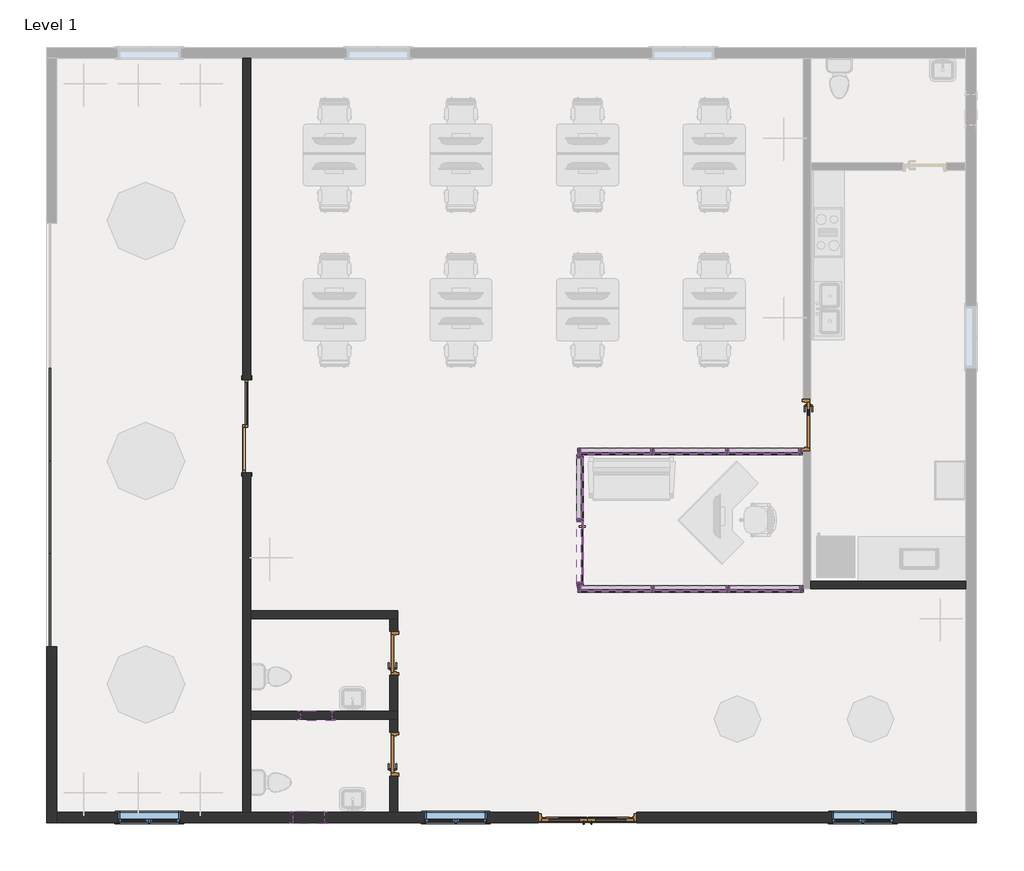
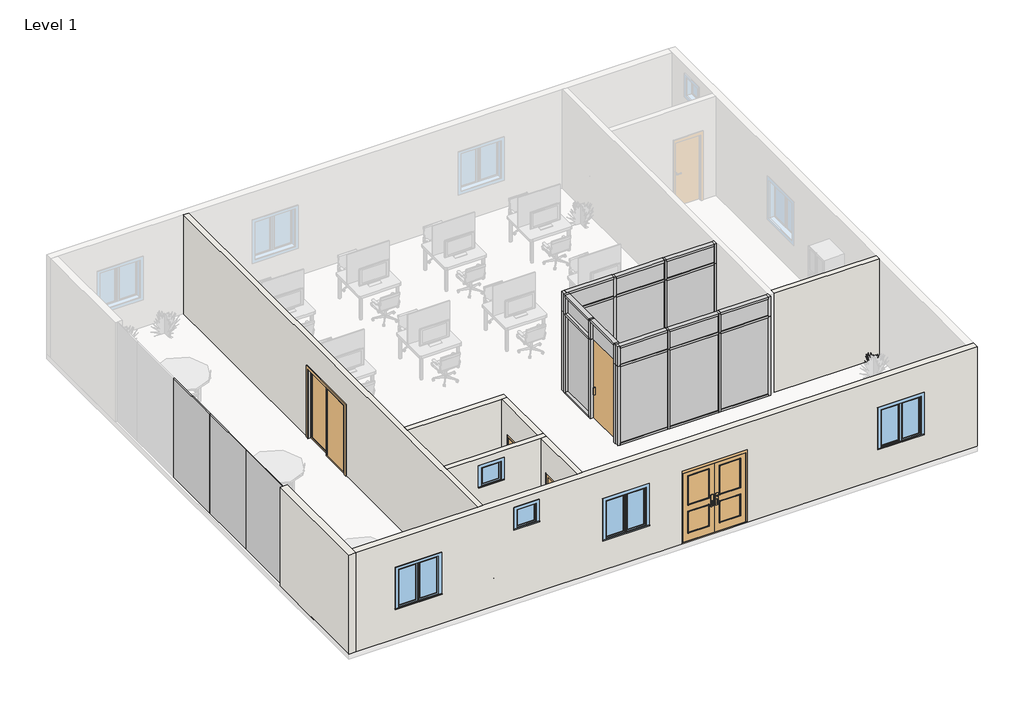
# One storey, part 1 of 2: 44 members, 18 plates, 8 walls, 6 doors, 5 windows.
"""IFC4 building model written with IfcOpenShell, lengths in millimetres."""

from ifc_helpers import new_model, si_unit, frame, origin, origin_with_axes, place, context, project, spatial, polyline, outline, extrude, faceted_brep, transform, mapped, element, save
from components import door_curtain_wall_single_glass_door_curtain_wall_single_8a977710, door_b43bda57, door_6260e01d, door_549a8064, door_95a5efb1, door_bb4af967, door_1568ef6f, member_79cc3911, member_243ec899, member_4dc7c44e, member_7022ac76, member_f0fea5a5, member_6e77e263, member_ee409385, member_47bfaf8a, member_e1cf819f, member_4b717c4e, member_f7ba7797, member_7354043d, member_7f33020a, member_c704a0f7, system_panel_glazed_acd1c6f8, system_panel_glazed_c99c457a, system_panel_glazed_58f29689, system_panel_glazed_e44632c1, system_panel_glazed_4b614736, system_panel_glazed_1dbb284f, system_panel_glazed_fd42546f, system_panel_glazed_94232cd9, system_panel_glazed_3d3fe78f, system_panel_glazed_8a2d2adf, system_panel_glazed_e91e0514, system_panel_glazed_5475d124, window_0862ab64, window_e41d21a6, window_3d781103

model = new_model("IFC4")

# Units and contexts
model_context = context("Model", 3, world=origin())
ifc_project = project(units=[si_unit("LENGTHUNIT", "METRE", prefix="MILLI")], contexts=[model_context])

# Site, building, storey
site = spatial("IfcSite", under=ifc_project)
building = spatial("IfcBuilding", under=site)
storey = spatial("IfcBuildingStorey", under=building, Name="Level 1", Elevation=0.0)

# Doors
placement = place(None, origin())
door_curtain_wall_single_glass_door_curtain_wall_single_shape = door_curtain_wall_single_glass_door_curtain_wall_single_8a977710(model_context)
element("IfcDoor", 1, ObjectType="Door-Curtain-Wall-Single-Glass : Door-Curtain-Wall-Single-Glass", at=placement, inside=storey, context=model_context, shape_type="MappedRepresentation", body=[
    mapped(door_curtain_wall_single_glass_door_curtain_wall_single_shape, transform((-9796.2738969, -3317.2711575, 0.0), x_axis=(0.0, -1.0, 0.0), y_axis=(1.0, 0.0, 0.0), z_axis=(0.0, 0.0, 1.0))),
])
door_shape = door_b43bda57(model_context)
element("IfcDoor", 2, ObjectType="Door-Double-Sliding : 72\" x 84\"", at=placement, inside=storey, context=model_context, shape_type="MappedRepresentation", body=[
    mapped(door_shape, transform((-16228.8238969, -839.1836575, 0.0), x_axis=(0.0, 1.0, 0.0), y_axis=(-1.0, 0.0, 0.0), z_axis=(0.0, 0.0, 1.0))),
])
door_2_shape = door_6260e01d(model_context)
door_3_shape = door_549a8064(model_context)
door_4_shape = door_95a5efb1(model_context)
element("IfcDoor", 3, ObjectType="Door-Exterior-Double-Two_Lite : 72\" x 84\"", at=placement, inside=storey, context=model_context, shape_type="MappedRepresentation", body=[
    mapped(door_2_shape, transform((-9650.2238969, -8529.0336575, 0.0), x_axis=(-1.0, 0.0, 0.0), y_axis=(0.0, -1.0, 0.0), z_axis=(0.0, 0.0, 1.0))),
    mapped(door_3_shape, transform((-9650.2238969, -8529.0336575, 0.0), x_axis=(-1.0, 0.0, 0.0), y_axis=(0.0, -1.0, 0.0), z_axis=(0.0, 0.0, 1.0))),
    mapped(door_4_shape, transform((-9650.2238969, -8529.0336575, 0.0), x_axis=(-1.0, 0.0, 0.0), y_axis=(0.0, -1.0, 0.0), z_axis=(0.0, 0.0, 1.0))),
])
door_5_shape = door_bb4af967(model_context)
element("IfcDoor", 4, ObjectType="Door-Passage-Single-Flush : 30\" x 80\"", at=placement, inside=storey, context=model_context, shape_type="MappedRepresentation", body=[
    mapped(door_5_shape, transform((-13453.8738969, -5309.5836575, 0.0), x_axis=(0.0, 1.0, 0.0), y_axis=(-1.0, 0.0, 0.0), z_axis=(0.0, 0.0, 1.0))),
])
element("IfcDoor", 5, ObjectType="Door-Passage-Single-Flush : 30\" x 80\"", at=placement, inside=storey, context=model_context, shape_type="MappedRepresentation", body=[
    mapped(door_5_shape, transform((-13453.8738969, -7290.7836575, 0.0), x_axis=(0.0, 1.0, 0.0), y_axis=(-1.0, 0.0, 0.0), z_axis=(0.0, 0.0, 1.0))),
])
door_6_shape = door_1568ef6f(model_context)
element("IfcDoor", 6, ObjectType="Door-Passage-Single-Two_Lite_Narrow : 36\" x 84\"", at=placement, inside=storey, context=model_context, shape_type="MappedRepresentation", body=[
    mapped(door_6_shape, transform((-5338.5738969, -813.7836575, 0.0), x_axis=(0.0, -1.0, 0.0), y_axis=(1.0, 0.0, 0.0), z_axis=(0.0, 0.0, 1.0))),
])

# Members
member_shape = member_79cc3911(model_context)
element("IfcMember", 7, ObjectType="Rectangular Mullion : 2.5\" x 5\" rectangular", at=placement, inside=storey, context=model_context, shape_type="MappedRepresentation", body=[
    mapped(member_shape, transform((-9783.5738969, -1340.8336575, 3048.0), x_axis=(0.0, 0.0, 1.0), y_axis=(0.0, 1.0, 0.0), z_axis=(-1.0, 0.0, 0.0))),
])
element("IfcMember", 8, ObjectType="Rectangular Mullion : 2.5\" x 5\" rectangular", at=placement, inside=storey, context=model_context, shape_type="MappedRepresentation", body=[
    mapped(member_shape, transform((-6868.9238969, -1340.8336575, 3048.0), x_axis=(0.0, 0.0, 1.0), y_axis=(0.0, 1.0, 0.0), z_axis=(-1.0, 0.0, 0.0))),
])
member_2_shape = member_243ec899(model_context)
element("IfcMember", 9, ObjectType="Rectangular Mullion : 2.5\" x 5\" rectangular", at=placement, inside=storey, context=model_context, shape_type="MappedRepresentation", body=[
    mapped(member_2_shape, transform((-8342.1238969, -1340.8336575, 3048.0), x_axis=(0.0, 0.0, 1.0), y_axis=(0.0, 1.0, 0.0), z_axis=(-1.0, 0.0, 0.0))),
])
element("IfcMember", 10, ObjectType="Rectangular Mullion : 2.5\" x 5\" rectangular", at=placement, inside=storey, context=model_context, shape_type="MappedRepresentation", body=[
    mapped(member_shape, transform((-5490.9738969, -1340.8336575, 0.0), x_axis=(0.0, 0.0, -1.0), y_axis=(0.0, 1.0, 0.0), z_axis=(1.0, 0.0, 0.0))),
])
element("IfcMember", 11, ObjectType="Rectangular Mullion : 2.5\" x 5\" rectangular", at=placement, inside=storey, context=model_context, shape_type="MappedRepresentation", body=[
    mapped(member_shape, transform((-8405.6238969, -1340.8336575, 0.0), x_axis=(0.0, 0.0, -1.0), y_axis=(0.0, 1.0, 0.0), z_axis=(1.0, 0.0, 0.0))),
])
element("IfcMember", 12, ObjectType="Rectangular Mullion : 2.5\" x 5\" rectangular", at=placement, inside=storey, context=model_context, shape_type="MappedRepresentation", body=[
    mapped(member_2_shape, transform((-6932.4238969, -1340.8336575, 0.0), x_axis=(0.0, 0.0, -1.0), y_axis=(0.0, 1.0, 0.0), z_axis=(1.0, 0.0, 0.0))),
])
member_3_shape = member_4dc7c44e(model_context)
element("IfcMember", 13, ObjectType="Rectangular Mullion : 2.5\" x 5\" rectangular", at=placement, inside=storey, context=model_context, shape_type="MappedRepresentation", body=[
    mapped(member_3_shape, transform((-6868.9238969, -1340.8336575, 2438.4), x_axis=(0.0, 0.0, 1.0), y_axis=(0.0, 1.0, 0.0), z_axis=(-1.0, 0.0, 0.0))),
])
element("IfcMember", 14, ObjectType="Rectangular Mullion : 2.5\" x 5\" rectangular", at=placement, inside=storey, context=model_context, shape_type="MappedRepresentation", body=[
    mapped(member_3_shape, transform((-9783.5738969, -1340.8336575, 2438.4), x_axis=(0.0, 0.0, 1.0), y_axis=(0.0, 1.0, 0.0), z_axis=(-1.0, 0.0, 0.0))),
])
member_4_shape = member_7022ac76(model_context)
element("IfcMember", 15, ObjectType="Rectangular Mullion : 2.5\" x 5\" rectangular", at=placement, inside=storey, context=model_context, shape_type="MappedRepresentation", body=[
    mapped(member_4_shape, transform((-8342.1238969, -1340.8336575, 2438.4), x_axis=(0.0, 0.0, 1.0), y_axis=(0.0, 1.0, 0.0), z_axis=(-1.0, 0.0, 0.0))),
])
member_5_shape = member_f0fea5a5(model_context)
element("IfcMember", 16, ObjectType="Rectangular Mullion : 2.5\" x 5\" rectangular", at=placement, inside=storey, context=model_context, shape_type="MappedRepresentation", body=[
    mapped(member_5_shape, transform((-6900.6738969, -1340.8336575, 0.0), x_axis=(-1.0, 0.0, 0.0), y_axis=(0.0, 1.0, 0.0), z_axis=(0.0, 0.0, -1.0))),
])
element("IfcMember", 17, ObjectType="Rectangular Mullion : 2.5\" x 5\" rectangular", at=placement, inside=storey, context=model_context, shape_type="MappedRepresentation", body=[
    mapped(member_5_shape, transform((-8373.8738969, -1340.8336575, 0.0), x_axis=(-1.0, 0.0, 0.0), y_axis=(0.0, 1.0, 0.0), z_axis=(0.0, 0.0, -1.0))),
])
element("IfcMember", 18, ObjectType="Rectangular Mullion : 2.5\" x 5\" rectangular", at=placement, inside=storey, context=model_context, shape_type="MappedRepresentation", body=[
    mapped(member_5_shape, transform((-6887.9738969, -4039.5836575, 0.0), x_axis=(-1.0, 0.0, 0.0), y_axis=(0.0, 1.0, 0.0), z_axis=(0.0, 0.0, -1.0))),
])
element("IfcMember", 19, ObjectType="Rectangular Mullion : 2.5\" x 5\" rectangular", at=placement, inside=storey, context=model_context, shape_type="MappedRepresentation", body=[
    mapped(member_5_shape, transform((-8367.5238969, -4039.5836575, 0.0), x_axis=(-1.0, 0.0, 0.0), y_axis=(0.0, 1.0, 0.0), z_axis=(0.0, 0.0, -1.0))),
])
element("IfcMember", 20, ObjectType="Rectangular Mullion : 2.5\" x 5\" rectangular", at=placement, inside=storey, context=model_context, shape_type="MappedRepresentation", body=[
    mapped(member_5_shape, transform((-9796.2738969, -2690.2086575, 0.0), x_axis=(0.0, -1.0, 0.0), y_axis=(-1.0, 0.0, 0.0), z_axis=(0.0, 0.0, -1.0))),
])
member_6_shape = member_6e77e263(model_context)
element("IfcMember", 21, ObjectType="Rectangular Mullion : 2.5\" x 5\" rectangular", at=placement, inside=storey, context=model_context, shape_type="MappedRepresentation", body=[
    mapped(member_6_shape, transform((-6900.6738969, -1340.8336575, 2438.4), x_axis=(-1.0, 0.0, 0.0), y_axis=(0.0, 1.0, 0.0), z_axis=(0.0, 0.0, -1.0))),
])
element("IfcMember", 22, ObjectType="Rectangular Mullion : 2.5\" x 5\" rectangular", at=placement, inside=storey, context=model_context, shape_type="MappedRepresentation", body=[
    mapped(member_6_shape, transform((-8373.8738969, -1340.8336575, 2438.4), x_axis=(-1.0, 0.0, 0.0), y_axis=(0.0, 1.0, 0.0), z_axis=(0.0, 0.0, -1.0))),
])
element("IfcMember", 23, ObjectType="Rectangular Mullion : 2.5\" x 5\" rectangular", at=placement, inside=storey, context=model_context, shape_type="MappedRepresentation", body=[
    mapped(member_6_shape, transform((-6887.9738969, -4039.5836575, 2438.4), x_axis=(-1.0, 0.0, 0.0), y_axis=(0.0, 1.0, 0.0), z_axis=(0.0, 0.0, -1.0))),
])
element("IfcMember", 24, ObjectType="Rectangular Mullion : 2.5\" x 5\" rectangular", at=placement, inside=storey, context=model_context, shape_type="MappedRepresentation", body=[
    mapped(member_6_shape, transform((-8367.5238969, -4039.5836575, 2438.4), x_axis=(-1.0, 0.0, 0.0), y_axis=(0.0, 1.0, 0.0), z_axis=(0.0, 0.0, -1.0))),
])
element("IfcMember", 25, ObjectType="Rectangular Mullion : 2.5\" x 5\" rectangular", at=placement, inside=storey, context=model_context, shape_type="MappedRepresentation", body=[
    mapped(member_6_shape, transform((-9796.2738969, -2690.2086575, 2438.4), x_axis=(0.0, -1.0, 0.0), y_axis=(-1.0, 0.0, 0.0), z_axis=(0.0, 0.0, -1.0))),
])
member_7_shape = member_ee409385(model_context)
element("IfcMember", 26, ObjectType="Rectangular Mullion : 2.5\" x 5\" rectangular", at=placement, inside=storey, context=model_context, shape_type="MappedRepresentation", body=[
    mapped(member_7_shape, transform((-9847.0738969, -1340.8336575, 0.0), x_axis=(-1.0, 0.0, 0.0), y_axis=(0.0, 1.0, 0.0), z_axis=(0.0, 0.0, -1.0))),
])
element("IfcMember", 27, ObjectType="Rectangular Mullion : 2.5\" x 5\" rectangular", at=placement, inside=storey, context=model_context, shape_type="MappedRepresentation", body=[
    mapped(member_7_shape, transform((-9847.0738969, -4039.5836575, 0.0), x_axis=(-1.0, 0.0, 0.0), y_axis=(0.0, 1.0, 0.0), z_axis=(0.0, 0.0, -1.0))),
])
member_8_shape = member_47bfaf8a(model_context)
element("IfcMember", 28, ObjectType="Rectangular Mullion : 2.5\" x 5\" rectangular", at=placement, inside=storey, context=model_context, shape_type="MappedRepresentation", body=[
    mapped(member_8_shape, transform((-9847.0738969, -1340.8336575, 2438.4), x_axis=(-1.0, 0.0, 0.0), y_axis=(0.0, 1.0, 0.0), z_axis=(0.0, 0.0, -1.0))),
])
element("IfcMember", 29, ObjectType="Rectangular Mullion : 2.5\" x 5\" rectangular", at=placement, inside=storey, context=model_context, shape_type="MappedRepresentation", body=[
    mapped(member_8_shape, transform((-9847.0738969, -4039.5836575, 2438.4), x_axis=(-1.0, 0.0, 0.0), y_axis=(0.0, 1.0, 0.0), z_axis=(0.0, 0.0, -1.0))),
])
element("IfcMember", 30, ObjectType="Rectangular Mullion : 2.5\" x 5\" rectangular", at=placement, inside=storey, context=model_context, shape_type="MappedRepresentation", body=[
    mapped(member_8_shape, transform((-5427.4738969, -1340.8336575, 3048.0), x_axis=(1.0, 0.0, 0.0), y_axis=(0.0, 1.0, 0.0), z_axis=(0.0, 0.0, 1.0))),
])
element("IfcMember", 31, ObjectType="Rectangular Mullion : 2.5\" x 5\" rectangular", at=placement, inside=storey, context=model_context, shape_type="MappedRepresentation", body=[
    mapped(member_8_shape, transform((-5408.4238969, -4039.5836575, 3048.0), x_axis=(1.0, 0.0, 0.0), y_axis=(0.0, 1.0, 0.0), z_axis=(0.0, 0.0, 1.0))),
])
element("IfcMember", 32, ObjectType="Rectangular Mullion : 2.5\" x 5\" rectangular", at=placement, inside=storey, context=model_context, shape_type="MappedRepresentation", body=[
    mapped(member_8_shape, transform((-9796.2738969, -1404.3336575, 3048.0), x_axis=(0.0, 1.0, 0.0), y_axis=(-1.0, 0.0, 0.0), z_axis=(0.0, 0.0, 1.0))),
])
element("IfcMember", 33, ObjectType="Rectangular Mullion : 2.5\" x 5\" rectangular", at=placement, inside=storey, context=model_context, shape_type="MappedRepresentation", body=[
    mapped(member_7_shape, transform((-5427.4738969, -1340.8336575, 2438.4), x_axis=(1.0, 0.0, 0.0), y_axis=(0.0, 1.0, 0.0), z_axis=(0.0, 0.0, 1.0))),
])
element("IfcMember", 34, ObjectType="Rectangular Mullion : 2.5\" x 5\" rectangular", at=placement, inside=storey, context=model_context, shape_type="MappedRepresentation", body=[
    mapped(member_7_shape, transform((-5408.4238969, -4039.5836575, 2438.4), x_axis=(1.0, 0.0, 0.0), y_axis=(0.0, 1.0, 0.0), z_axis=(0.0, 0.0, 1.0))),
])
element("IfcMember", 35, ObjectType="Rectangular Mullion : 2.5\" x 5\" rectangular", at=placement, inside=storey, context=model_context, shape_type="MappedRepresentation", body=[
    mapped(member_7_shape, transform((-9796.2738969, -1404.3336575, 2438.4), x_axis=(0.0, 1.0, 0.0), y_axis=(-1.0, 0.0, 0.0), z_axis=(0.0, 0.0, 1.0))),
])
member_9_shape = member_e1cf819f(model_context)
element("IfcMember", 36, ObjectType="Rectangular Mullion : 2.5\" x 5\" rectangular", at=placement, inside=storey, context=model_context, shape_type="MappedRepresentation", body=[
    mapped(member_9_shape, transform((-9783.5738969, -4039.5836575, 3048.0), x_axis=(0.0, 0.0, 1.0), y_axis=(0.0, 1.0, 0.0), z_axis=(-1.0, 0.0, 0.0))),
])
element("IfcMember", 37, ObjectType="Rectangular Mullion : 2.5\" x 5\" rectangular", at=placement, inside=storey, context=model_context, shape_type="MappedRepresentation", body=[
    mapped(member_9_shape, transform((-6856.2238969, -4039.5836575, 3048.0), x_axis=(0.0, 0.0, 1.0), y_axis=(0.0, 1.0, 0.0), z_axis=(-1.0, 0.0, 0.0))),
])
member_10_shape = member_4b717c4e(model_context)
element("IfcMember", 38, ObjectType="Rectangular Mullion : 2.5\" x 5\" rectangular", at=placement, inside=storey, context=model_context, shape_type="MappedRepresentation", body=[
    mapped(member_10_shape, transform((-8335.7738969, -4039.5836575, 3048.0), x_axis=(0.0, 0.0, 1.0), y_axis=(0.0, 1.0, 0.0), z_axis=(-1.0, 0.0, 0.0))),
])
element("IfcMember", 39, ObjectType="Rectangular Mullion : 2.5\" x 5\" rectangular", at=placement, inside=storey, context=model_context, shape_type="MappedRepresentation", body=[
    mapped(member_9_shape, transform((-5471.9238969, -4039.5836575, 0.0), x_axis=(0.0, 0.0, -1.0), y_axis=(0.0, 1.0, 0.0), z_axis=(1.0, 0.0, 0.0))),
])
element("IfcMember", 40, ObjectType="Rectangular Mullion : 2.5\" x 5\" rectangular", at=placement, inside=storey, context=model_context, shape_type="MappedRepresentation", body=[
    mapped(member_9_shape, transform((-8399.2738969, -4039.5836575, 0.0), x_axis=(0.0, 0.0, -1.0), y_axis=(0.0, 1.0, 0.0), z_axis=(1.0, 0.0, 0.0))),
])
element("IfcMember", 41, ObjectType="Rectangular Mullion : 2.5\" x 5\" rectangular", at=placement, inside=storey, context=model_context, shape_type="MappedRepresentation", body=[
    mapped(member_10_shape, transform((-6919.7238969, -4039.5836575, 0.0), x_axis=(0.0, 0.0, -1.0), y_axis=(0.0, 1.0, 0.0), z_axis=(1.0, 0.0, 0.0))),
])
member_11_shape = member_f7ba7797(model_context)
element("IfcMember", 42, ObjectType="Rectangular Mullion : 2.5\" x 5\" rectangular", at=placement, inside=storey, context=model_context, shape_type="MappedRepresentation", body=[
    mapped(member_11_shape, transform((-6856.2238969, -4039.5836575, 2438.4), x_axis=(0.0, 0.0, 1.0), y_axis=(0.0, 1.0, 0.0), z_axis=(-1.0, 0.0, 0.0))),
])
element("IfcMember", 43, ObjectType="Rectangular Mullion : 2.5\" x 5\" rectangular", at=placement, inside=storey, context=model_context, shape_type="MappedRepresentation", body=[
    mapped(member_11_shape, transform((-9783.5738969, -4039.5836575, 2438.4), x_axis=(0.0, 0.0, 1.0), y_axis=(0.0, 1.0, 0.0), z_axis=(-1.0, 0.0, 0.0))),
])
member_12_shape = member_7354043d(model_context)
element("IfcMember", 44, ObjectType="Rectangular Mullion : 2.5\" x 5\" rectangular", at=placement, inside=storey, context=model_context, shape_type="MappedRepresentation", body=[
    mapped(member_12_shape, transform((-8335.7738969, -4039.5836575, 2438.4), x_axis=(0.0, 0.0, 1.0), y_axis=(0.0, 1.0, 0.0), z_axis=(-1.0, 0.0, 0.0))),
])
member_13_shape = member_7f33020a(model_context)
element("IfcMember", 45, ObjectType="Rectangular Mullion : 2.5\" x 5\" rectangular", at=placement, inside=storey, context=model_context, shape_type="MappedRepresentation", body=[
    mapped(member_13_shape, transform((-9796.2738969, -3912.5836575, 3048.0), x_axis=(0.0, 0.0, 1.0), y_axis=(-1.0, 0.0, 0.0), z_axis=(0.0, -1.0, 0.0))),
])
element("IfcMember", 46, ObjectType="Rectangular Mullion : 2.5\" x 5\" rectangular", at=placement, inside=storey, context=model_context, shape_type="MappedRepresentation", body=[
    mapped(member_13_shape, transform((-9796.2738969, -2658.4586575, 3048.0), x_axis=(0.0, 0.0, 1.0), y_axis=(-1.0, 0.0, 0.0), z_axis=(0.0, -1.0, 0.0))),
])
element("IfcMember", 47, ObjectType="Rectangular Mullion : 2.5\" x 5\" rectangular", at=placement, inside=storey, context=model_context, shape_type="MappedRepresentation", body=[
    mapped(member_13_shape, transform((-9796.2738969, -1467.8336575, 0.0), x_axis=(0.0, 0.0, -1.0), y_axis=(-1.0, 0.0, 0.0), z_axis=(0.0, 1.0, 0.0))),
])
member_14_shape = member_c704a0f7(model_context)
element("IfcMember", 48, ObjectType="Rectangular Mullion : 2.5\" x 5\" rectangular", at=placement, inside=storey, context=model_context, shape_type="MappedRepresentation", body=[
    mapped(member_14_shape, transform((-9796.2738969, -2658.4586575, 2438.4), x_axis=(0.0, 0.0, 1.0), y_axis=(-1.0, 0.0, 0.0), z_axis=(0.0, -1.0, 0.0))),
])
element("IfcMember", 49, ObjectType="Rectangular Mullion : 2.5\" x 5\" rectangular", at=placement, inside=storey, context=model_context, shape_type="MappedRepresentation", body=[
    mapped(member_8_shape, transform((-9796.2738969, -3976.0836575, 2438.4), x_axis=(0.0, -1.0, 0.0), y_axis=(-1.0, 0.0, 0.0), z_axis=(0.0, 0.0, -1.0))),
])
element("IfcMember", 50, ObjectType="Rectangular Mullion : 2.5\" x 5\" rectangular", at=placement, inside=storey, context=model_context, shape_type="MappedRepresentation", body=[
    mapped(member_7_shape, transform((-9796.2738969, -3976.0836575, 0.0), x_axis=(0.0, -1.0, 0.0), y_axis=(-1.0, 0.0, 0.0), z_axis=(0.0, 0.0, -1.0))),
])

# Plates
system_panel_glazed_shape = system_panel_glazed_acd1c6f8(model_context)
element("IfcPlate", 51, ObjectType="System Panel : Glazed", at=placement, inside=storey, context=model_context, shape_type="MappedRepresentation", body=[
    mapped(system_panel_glazed_shape, transform((-20191.2238969, -4268.1836575, 0.0), x_axis=(0.0, 1.0, 0.0), y_axis=(-1.0, 0.0, 0.0), z_axis=(0.0, 0.0, 1.0))),
])
element("IfcPlate", 52, ObjectType="System Panel : Glazed", at=placement, inside=storey, context=model_context, shape_type="MappedRepresentation", body=[
    mapped(system_panel_glazed_shape, transform((-20191.2238969, -2439.3836575, 0.0), x_axis=(0.0, 1.0, 0.0), y_axis=(-1.0, 0.0, 0.0), z_axis=(0.0, 0.0, 1.0))),
])
element("IfcPlate", 53, ObjectType="System Panel : Glazed", at=placement, inside=storey, context=model_context, shape_type="MappedRepresentation", body=[
    mapped(system_panel_glazed_shape, transform((-20191.2238969, -610.5836575, 0.0), x_axis=(0.0, 1.0, 0.0), y_axis=(-1.0, 0.0, 0.0), z_axis=(0.0, 0.0, 1.0))),
])
system_panel_glazed_2_shape = system_panel_glazed_c99c457a(model_context)
element("IfcPlate", 54, ObjectType="System Panel : Glazed", at=placement, inside=storey, context=model_context, shape_type="MappedRepresentation", body=[
    mapped(system_panel_glazed_2_shape, transform((-6179.9488969, -1340.8336575, 63.5), x_axis=(-1.0, 0.0, 0.0), y_axis=(0.0, -1.0, 0.0), z_axis=(0.0, 0.0, 1.0))),
])
element("IfcPlate", 55, ObjectType="System Panel : Glazed", at=placement, inside=storey, context=model_context, shape_type="MappedRepresentation", body=[
    mapped(system_panel_glazed_2_shape, transform((-9094.5988969, -1340.8336575, 63.5), x_axis=(-1.0, 0.0, 0.0), y_axis=(0.0, -1.0, 0.0), z_axis=(0.0, 0.0, 1.0))),
])
system_panel_glazed_3_shape = system_panel_glazed_58f29689(model_context)
element("IfcPlate", 56, ObjectType="System Panel : Glazed", at=placement, inside=storey, context=model_context, shape_type="MappedRepresentation", body=[
    mapped(system_panel_glazed_3_shape, transform((-7637.2738969, -1340.8336575, 63.5), x_axis=(-1.0, 0.0, 0.0), y_axis=(0.0, -1.0, 0.0), z_axis=(0.0, 0.0, 1.0))),
])
system_panel_glazed_4_shape = system_panel_glazed_e44632c1(model_context)
element("IfcPlate", 57, ObjectType="System Panel : Glazed", at=placement, inside=storey, context=model_context, shape_type="MappedRepresentation", body=[
    mapped(system_panel_glazed_4_shape, transform((-6179.9488969, -1340.8336575, 2470.15), x_axis=(-1.0, 0.0, 0.0), y_axis=(0.0, -1.0, 0.0), z_axis=(0.0, 0.0, 1.0))),
])
element("IfcPlate", 58, ObjectType="System Panel : Glazed", at=placement, inside=storey, context=model_context, shape_type="MappedRepresentation", body=[
    mapped(system_panel_glazed_4_shape, transform((-9094.5988969, -1340.8336575, 2470.15), x_axis=(-1.0, 0.0, 0.0), y_axis=(0.0, -1.0, 0.0), z_axis=(0.0, 0.0, 1.0))),
])
system_panel_glazed_5_shape = system_panel_glazed_4b614736(model_context)
element("IfcPlate", 59, ObjectType="System Panel : Glazed", at=placement, inside=storey, context=model_context, shape_type="MappedRepresentation", body=[
    mapped(system_panel_glazed_5_shape, transform((-7637.2738969, -1340.8336575, 2470.15), x_axis=(-1.0, 0.0, 0.0), y_axis=(0.0, -1.0, 0.0), z_axis=(0.0, 0.0, 1.0))),
])
system_panel_glazed_6_shape = system_panel_glazed_1dbb284f(model_context)
element("IfcPlate", 60, ObjectType="System Panel : Glazed", at=placement, inside=storey, context=model_context, shape_type="MappedRepresentation", body=[
    mapped(system_panel_glazed_6_shape, transform((-6164.0738969, -4039.5836575, 63.5), x_axis=(-1.0, 0.0, 0.0), y_axis=(0.0, -1.0, 0.0), z_axis=(0.0, 0.0, 1.0))),
])
element("IfcPlate", 61, ObjectType="System Panel : Glazed", at=placement, inside=storey, context=model_context, shape_type="MappedRepresentation", body=[
    mapped(system_panel_glazed_6_shape, transform((-9091.4238969, -4039.5836575, 63.5), x_axis=(-1.0, 0.0, 0.0), y_axis=(0.0, -1.0, 0.0), z_axis=(0.0, 0.0, 1.0))),
])
system_panel_glazed_7_shape = system_panel_glazed_fd42546f(model_context)
element("IfcPlate", 62, ObjectType="System Panel : Glazed", at=placement, inside=storey, context=model_context, shape_type="MappedRepresentation", body=[
    mapped(system_panel_glazed_7_shape, transform((-7627.7488969, -4039.5836575, 63.5), x_axis=(-1.0, 0.0, 0.0), y_axis=(0.0, -1.0, 0.0), z_axis=(0.0, 0.0, 1.0))),
])
system_panel_glazed_8_shape = system_panel_glazed_94232cd9(model_context)
element("IfcPlate", 63, ObjectType="System Panel : Glazed", at=placement, inside=storey, context=model_context, shape_type="MappedRepresentation", body=[
    mapped(system_panel_glazed_8_shape, transform((-6164.0738969, -4039.5836575, 2470.15), x_axis=(-1.0, 0.0, 0.0), y_axis=(0.0, -1.0, 0.0), z_axis=(0.0, 0.0, 1.0))),
])
element("IfcPlate", 64, ObjectType="System Panel : Glazed", at=placement, inside=storey, context=model_context, shape_type="MappedRepresentation", body=[
    mapped(system_panel_glazed_8_shape, transform((-9091.4238969, -4039.5836575, 2470.15), x_axis=(-1.0, 0.0, 0.0), y_axis=(0.0, -1.0, 0.0), z_axis=(0.0, 0.0, 1.0))),
])
system_panel_glazed_9_shape = system_panel_glazed_3d3fe78f(model_context)
element("IfcPlate", 65, ObjectType="System Panel : Glazed", at=placement, inside=storey, context=model_context, shape_type="MappedRepresentation", body=[
    mapped(system_panel_glazed_9_shape, transform((-7627.7488969, -4039.5836575, 2470.15), x_axis=(-1.0, 0.0, 0.0), y_axis=(0.0, -1.0, 0.0), z_axis=(0.0, 0.0, 1.0))),
])
system_panel_glazed_10_shape = system_panel_glazed_8a2d2adf(model_context)
element("IfcPlate", 66, ObjectType="System Panel : Glazed", at=placement, inside=storey, context=model_context, shape_type="MappedRepresentation", body=[
    mapped(system_panel_glazed_10_shape, transform((-9796.2738969, -2063.1461575, 63.5), x_axis=(0.0, -1.0, 0.0), y_axis=(1.0, 0.0, 0.0), z_axis=(0.0, 0.0, 1.0))),
])
system_panel_glazed_11_shape = system_panel_glazed_e91e0514(model_context)
element("IfcPlate", 67, ObjectType="System Panel : Glazed", at=placement, inside=storey, context=model_context, shape_type="MappedRepresentation", body=[
    mapped(system_panel_glazed_11_shape, transform((-9796.2738969, -2063.1461575, 2470.15), x_axis=(0.0, -1.0, 0.0), y_axis=(1.0, 0.0, 0.0), z_axis=(0.0, 0.0, 1.0))),
])
system_panel_glazed_12_shape = system_panel_glazed_5475d124(model_context)
element("IfcPlate", 68, ObjectType="System Panel : Glazed", at=placement, inside=storey, context=model_context, shape_type="MappedRepresentation", body=[
    mapped(system_panel_glazed_12_shape, transform((-9796.2738969, -3317.2711575, 2438.4), x_axis=(0.0, -1.0, 0.0), y_axis=(1.0, 0.0, 0.0), z_axis=(0.0, 0.0, 1.0))),
])

# Walls
element("IfcWall", 69, ObjectType="Generic - 6\"", at=placement, inside=storey, context=model_context, shape_type="Brep", body=[
    faceted_brep([(-16432.0238969, 6399.8163425, 0.0), (-16432.0238969, 75.2163425, 0.0), (-16432.0238969, 75.2163425, 2133.6), (-16432.0238969, -1753.5836575, 2133.6), (-16432.0238969, -1753.5836575, 0.0), (-16432.0238969, -8433.7836575, 0.0), (-16432.0238969, -8433.7836575, 3048.0), (-16432.0238969, 6399.8163425, 3048.0), (-16279.6238969, 75.2163425, 2133.6), (-16279.6238969, 75.2163425, 0.0), (-16279.6238969, 6399.8163425, 0.0), (-16279.6238969, 6399.8163425, 3048.0), (-16279.6238969, -4471.3836575, 3048.0), (-16279.6238969, -4623.7836575, 3048.0), (-16279.6238969, -6452.5836575, 3048.0), (-16279.6238969, -6604.9836575, 3048.0), (-16279.6238969, -8433.7836575, 3048.0), (-16279.6238969, -8433.7836575, 0.0), (-16279.6238969, -6604.9836575, 0.0), (-16279.6238969, -6452.5836575, 0.0), (-16279.6238969, -4623.7836575, 0.0), (-16279.6238969, -4471.3836575, 0.0), (-16279.6238969, -1753.5836575, 0.0), (-16279.6238969, -1753.5836575, 2133.6)], [[[0, 1, 2, 3, 4, 5, 6, 7]], [[8, 9, 10, 11, 12, 13, 14, 15, 16, 17, 18, 19, 20, 21, 22, 23]], [[10, 9, 1, 0]], [[22, 21, 20, 19, 18, 17, 5, 4]], [[7, 6, 16, 15, 14, 13, 12, 11]], [[0, 7, 11, 10]], [[6, 5, 17, 16]], [[4, 3, 23, 22]], [[2, 1, 9, 8]], [[3, 2, 8, 23]]]),
])
element("IfcWall", 70, ObjectType="Generic - 6\"", at=placement, inside=storey, context=model_context, shape_type="Brep", body=[
    faceted_brep([(-16279.6238969, -6604.9836575, 0.0), (-13536.4238969, -6604.9836575, 0.0), (-13384.0238969, -6604.9836575, 0.0), (-13384.0238969, -6604.9836575, 3048.0), (-13536.4238969, -6604.9836575, 3048.0), (-16279.6238969, -6604.9836575, 3048.0), (-15289.0238969, -6604.9836575, 2768.6), (-14679.4238969, -6604.9836575, 2768.6), (-14679.4238969, -6604.9836575, 2159.0), (-15289.0238969, -6604.9836575, 2159.0), (-16279.6238969, -6452.5836575, 0.0), (-16279.6238969, -6452.5836575, 3048.0), (-13536.4238969, -6452.5836575, 3048.0), (-13384.0238969, -6452.5836575, 3048.0), (-13384.0238969, -6452.5836575, 0.0), (-13536.4238969, -6452.5836575, 0.0), (-15289.0238969, -6452.5836575, 2768.6), (-15289.0238969, -6452.5836575, 2159.0), (-14679.4238969, -6452.5836575, 2159.0), (-14679.4238969, -6452.5836575, 2768.6)], [[[0, 1, 2, 3, 4, 5], [6, 7, 8, 9]], [[10, 11, 12, 13, 14, 15], [16, 17, 18, 19]], [[2, 1, 0, 10, 15, 14]], [[5, 4, 3, 13, 12, 11]], [[0, 5, 11, 10]], [[3, 2, 14, 13]], [[17, 16, 6, 9]], [[18, 17, 9, 8]], [[19, 18, 8, 7]], [[16, 19, 7, 6]]]),
])
element("IfcWall", 71, ObjectType="Generic - 6\"", at=placement, inside=storey, context=model_context, shape_type="SweptSolid", body=[
    extrude(outline(polyline([(-8433.7836575, 3048.0), (-6604.9836575, 3048.0), (-6604.9836575, 0.0), (-6858.9836575, 0.0), (-6858.9836575, 2133.6), (-7722.5836575, 2133.6), (-7722.5836575, 0.0), (-8433.7836575, 0.0), (-8433.7836575, 3048.0)])), frame((-13536.4238969, 0.0, 0.0), z_axis=(1.0, 0.0, 0.0), x_axis=(0.0, 1.0, 0.0)), (0.0, 0.0, 1.0), 152.4),
])
element("IfcWall", 72, ObjectType="Generic - 6\"", at=placement, inside=storey, context=model_context, shape_type="Brep", body=[
    faceted_brep([(-16279.6238969, -4623.7836575, 0.0), (-13536.4238969, -4623.7836575, 0.0), (-13384.0238969, -4623.7836575, 0.0), (-13384.0238969, -4623.7836575, 3048.0), (-13536.4238969, -4623.7836575, 3048.0), (-16279.6238969, -4623.7836575, 3048.0), (-16279.6238969, -4471.3836575, 0.0), (-16279.6238969, -4471.3836575, 3048.0), (-13384.0238969, -4471.3836575, 3048.0), (-13384.0238969, -4471.3836575, 0.0)], [[[0, 1, 2, 3, 4, 5]], [[6, 7, 8, 9]], [[2, 1, 0, 6, 9]], [[5, 4, 3, 8, 7]], [[3, 2, 9, 8]], [[0, 5, 7, 6]]]),
])
element("IfcWall", 73, ObjectType="Generic - 6\"", at=placement, inside=storey, context=model_context, shape_type="SweptSolid", body=[
    extrude(outline(polyline([(-6452.5836575, 3048.0), (-4623.7836575, 3048.0), (-4623.7836575, 0.0), (-4877.7836575, 0.0), (-4877.7836575, 2133.6), (-5741.3836575, 2133.6), (-5741.3836575, 0.0), (-6452.5836575, 0.0), (-6452.5836575, 3048.0)])), frame((-13536.4238969, 0.0, 0.0), z_axis=(1.0, 0.0, 0.0), x_axis=(0.0, 1.0, 0.0)), (0.0, 0.0, 1.0), 152.4),
])
element("IfcWall", 74, ObjectType="Generic - 6\"", at=placement, inside=storey, context=model_context, shape_type="SweptSolid", body=[
    extrude(outline(polyline([(-2208.0238969, -4039.5836575), (-5256.0238969, -4039.5836575), (-5256.0238969, -3887.1836575), (-2208.0238969, -3887.1836575), (-2208.0238969, -4039.5836575)])), origin_with_axes(), (0.0, 0.0, 1.0), 3048.0),
])
element("IfcWall", 75, ObjectType="Generic - 8\"", at=placement, inside=storey, context=model_context, shape_type="Brep", body=[
    faceted_brep([(-20089.6238969, -8636.9836575, 0.0), (-20089.6238969, -8433.7836575, 0.0), (-20089.6238969, -5182.5836575, 0.0), (-20089.6238969, -5182.5836575, 3048.0), (-20089.6238969, -8433.7836575, 3048.0), (-20089.6238969, -8636.9836575, 3048.0), (-20292.8238969, -8636.9836575, 0.0), (-20292.8238969, -8636.9836575, 3048.0), (-20292.8238969, -5182.5836575, 3048.0), (-20292.8238969, -5182.5836575, 0.0)], [[[0, 1, 2, 3, 4, 5]], [[6, 7, 8, 9]], [[2, 1, 0, 6, 9]], [[3, 2, 9, 8]], [[5, 4, 3, 8, 7]], [[0, 5, 7, 6]]]),
])
element("IfcWall", 76, ObjectType="Generic - 8\"", at=placement, inside=storey, context=model_context, shape_type="Brep", body=[
    faceted_brep([(-20089.6238969, -8433.7836575, 3048.0), (-16432.0238969, -8433.7836575, 3048.0), (-16279.6238969, -8433.7836575, 3048.0), (-13536.4238969, -8433.7836575, 3048.0), (-13384.0238969, -8433.7836575, 3048.0), (-2208.0238969, -8433.7836575, 3048.0), (-2004.8238969, -8433.7836575, 3048.0), (-2004.8238969, -8433.7836575, 0.0), (-2208.0238969, -8433.7836575, 0.0), (-8685.0238969, -8433.7836575, 0.0), (-8685.0238969, -8433.7836575, 2235.2), (-10615.4238969, -8433.7836575, 2235.2), (-10615.4238969, -8433.7836575, 0.0), (-13384.0238969, -8433.7836575, 0.0), (-13536.4238969, -8433.7836575, 0.0), (-16279.6238969, -8433.7836575, 0.0), (-16432.0238969, -8433.7836575, 0.0), (-20089.6238969, -8433.7836575, 0.0), (-12850.6238969, -8433.7836575, 2133.6), (-12850.6238969, -8433.7836575, 914.4), (-11631.4238969, -8433.7836575, 914.4), (-11631.4238969, -8433.7836575, 2133.6), (-4849.6238969, -8433.7836575, 2133.6), (-4849.6238969, -8433.7836575, 914.4), (-3630.4238969, -8433.7836575, 914.4), (-3630.4238969, -8433.7836575, 2133.6), (-18883.1238969, -8433.7836575, 2133.6), (-18883.1238969, -8433.7836575, 914.4), (-17663.9238969, -8433.7836575, 914.4), (-17663.9238969, -8433.7836575, 2133.6), (-15441.4238969, -8433.7836575, 2768.6), (-15441.4238969, -8433.7836575, 2159.0), (-14831.8238969, -8433.7836575, 2159.0), (-14831.8238969, -8433.7836575, 2768.6), (-2004.8238969, -8636.9836575, 3048.0), (-20089.6238969, -8636.9836575, 3048.0), (-20089.6238969, -8636.9836575, 0.0), (-10615.4238969, -8636.9836575, 0.0), (-10615.4238969, -8636.9836575, 2235.2), (-8685.0238969, -8636.9836575, 2235.2), (-8685.0238969, -8636.9836575, 0.0), (-2004.8238969, -8636.9836575, 0.0), (-12850.6238969, -8636.9836575, 2133.6), (-11631.4238969, -8636.9836575, 2133.6), (-11631.4238969, -8636.9836575, 914.4), (-12850.6238969, -8636.9836575, 914.4), (-4849.6238969, -8636.9836575, 2133.6), (-3630.4238969, -8636.9836575, 2133.6), (-3630.4238969, -8636.9836575, 914.4), (-4849.6238969, -8636.9836575, 914.4), (-18883.1238969, -8636.9836575, 2133.6), (-17663.9238969, -8636.9836575, 2133.6), (-17663.9238969, -8636.9836575, 914.4), (-18883.1238969, -8636.9836575, 914.4), (-15441.4238969, -8636.9836575, 2768.6), (-14831.8238969, -8636.9836575, 2768.6), (-14831.8238969, -8636.9836575, 2159.0), (-15441.4238969, -8636.9836575, 2159.0)], [[[0, 1, 2, 3, 4, 5, 6, 7, 8, 9, 10, 11, 12, 13, 14, 15, 16, 17], [18, 19, 20, 21], [22, 23, 24, 25], [26, 27, 28, 29], [30, 31, 32, 33]], [[34, 35, 36, 37, 38, 39, 40, 41], [42, 43, 44, 45], [46, 47, 48, 49], [50, 51, 52, 53], [54, 55, 56, 57]], [[7, 41, 40, 9, 8]], [[36, 17, 16, 15, 14, 13, 12, 37]], [[6, 5, 4, 3, 2, 1, 0, 35, 34]], [[7, 6, 34, 41]], [[0, 17, 36, 35]], [[19, 18, 42, 45]], [[20, 19, 45, 44]], [[21, 20, 44, 43]], [[18, 21, 43, 42]], [[23, 22, 46, 49]], [[24, 23, 49, 48]], [[25, 24, 48, 47]], [[22, 25, 47, 46]], [[27, 26, 50, 53]], [[28, 27, 53, 52]], [[29, 28, 52, 51]], [[26, 29, 51, 50]], [[31, 30, 54, 57]], [[32, 31, 57, 56]], [[33, 32, 56, 55]], [[30, 33, 55, 54]], [[11, 38, 37, 12]], [[38, 11, 10, 39]], [[39, 10, 9, 40]]]),
])

# Windows
window_shape = window_0862ab64(model_context)
element("IfcWindow", 77, ObjectType="Casement Dbl with Trim : 48\" x 48\"", at=placement, inside=storey, context=model_context, shape_type="MappedRepresentation", body=[
    mapped(window_shape, transform((-12241.0238969, -8516.3336575, 0.0), x_axis=(-1.0, 0.0, 0.0), y_axis=(0.0, -1.0, 0.0), z_axis=(0.0, 0.0, 1.0))),
])
element("IfcWindow", 78, ObjectType="Casement Dbl with Trim : 48\" x 48\"", at=placement, inside=storey, context=model_context, shape_type="MappedRepresentation", body=[
    mapped(window_shape, transform((-4240.0238969, -8516.3336575, 0.0), x_axis=(-1.0, 0.0, 0.0), y_axis=(0.0, -1.0, 0.0), z_axis=(0.0, 0.0, 1.0))),
])
element("IfcWindow", 79, ObjectType="Casement Dbl with Trim : 48\" x 48\"", at=placement, inside=storey, context=model_context, shape_type="MappedRepresentation", body=[
    mapped(window_shape, transform((-18273.5238969, -8516.3336575, 0.0), x_axis=(-1.0, 0.0, 0.0), y_axis=(0.0, -1.0, 0.0), z_axis=(0.0, 0.0, 1.0))),
])
window_2_shape = window_e41d21a6(model_context)
element("IfcWindow", 80, ObjectType="Transom with Trim : 24\" x 24\"", at=placement, inside=storey, context=model_context, shape_type="MappedRepresentation", body=[
    mapped(window_2_shape, transform((-15174.7238969, -8535.3836575, 0.0), x_axis=(-1.0, 0.0, 0.0), y_axis=(0.0, -1.0, 0.0), z_axis=(0.0, 0.0, 1.0))),
])
window_3_shape = window_3d781103(model_context)
element("IfcWindow", 81, ObjectType="Transom with Trim : 24\" x 24\"", at=placement, inside=storey, context=model_context, shape_type="MappedRepresentation", body=[
    mapped(window_3_shape, transform((-15022.3238969, -6528.7836575, 0.0), x_axis=(-1.0, 0.0, 0.0), y_axis=(0.0, -1.0, 0.0), z_axis=(0.0, 0.0, 1.0))),
])

save(model, "model.ifc")

# Revit data of these elements
# Type "Door-Curtain-Wall-Single-Glass : Door-Curtain-Wall-Single-Glass"
#   Type Mark = "12"
#   Assembly Code = "B2030100"
#   Analytic Construction = "<None>"
#   Width [instance default] = 3' - 0"
#   Thermal Resistance (R) = 10.0000 (h·ft²·°F)/BTU
#   Swing Angle [instance default] = 90.00°
#   Heat Transfer Coefficient (U) = 0.1000 BTU/(h·ft²·°F)
#   Offset = 0' - 2"
#   Define Thermal Properties by = 1
#   Function = 1
#   Door Handle Material = Aluminum
#   Glazing = Glass
#   Visual Light Transmittance = 0
#   Solar Heat Gain Coefficient = 0
#   Construction Type Id = ""
# Type "Door-Double-Sliding : 72\" x 84\""
#   Type Mark = "9"
#   Construction Type Id = "opn-d45"
#   Assembly Code = "C1020"
#   Analytic Construction = "Wood frame, double glass door "
#   Thickness = 0' - 2"
#   Thermal Resistance (R) = 1.8150 (h·ft²·°F)/BTU
#   Heat Transfer Coefficient (U) = 0.5510 BTU/(h·ft²·°F)
#   Height = 7' - 0"
#   Rail Width = 0' - 2"
#   Stiles = 0' - 2"
#   Trim Projection Ext = 0' - 1"
#   Trim Projection Int = 0' - 1"
#   Trim Width = 0' - 3"
#   Width = 6' - 0"
#   Define Thermal Properties by = 1
#   Glazing = Glass
#   Panel Material = Wood - Birch - Solid Stained Light Low Gloss
#   Trim Material = Paint - Sienna
#   Visual Light Transmittance = 0
#   Solar Heat Gain Coefficient = 0
#   Function = (empty or 0)
#   Wall Closure = (empty or 0)
# Type "Door-Exterior-Double-Two_Lite : 72\" x 84\""
#   Type Mark = "8"
#   Assembly Code = "B2030100"
#   Analytic Construction = "Metal frame, double glass door"
#   Top Rail = 0' - 4 5/8"
#   Threshold Length [instance default] = 6' - 4"
#   Threshold Offset [instance default] = 0' - 0 1/2"
#   Thickness = 0' - 1 3/4"
#   Thermal Resistance (R) = 1.3794 (h·ft²·°F)/BTU
#   Swing Angle [instance default] = 90.00°
#   Strike Height = 3' - 4"
#   Stiles = 0' - 6"
#   SinglePanelWidth = 3' - 0"
#   Rough Width [instance default] = 6' - 4"
#   Rough Height [instance default] = 7' - 4"
#   MFOpeningHeight [instance default] = 0' - 4"
#   MFOpeningWidth [instance default] = 0' - 4"
#   Lock Rail = 0' - 8"
#   Inset Calculate [instance default] = 0' - 4"
#   Masonry Inset [instance default] = 0' - 1"
#   Height = 7' - 0"
#   Width = 6' - 0"
#   Heat Transfer Coefficient (U) = 0.7250 BTU/(h·ft²·°F)
#   Glass Thickness = 0' - 0 3/4"
#   Masonry Frame Depth = 0' - 5 3/4"
#   Bottom Rail = 0' - 10"
#   Threshold [instance default] = yes
#   Masonry Frame [instance default] = yes
#   Function = 1
#   Dry Wall Frame [instance default] = no
#   Threshold Material = none
#   Panic Bar Material = Metal - Stainless Steel
#   Panel Material = Metal - Painted - Grey
#   Glass Stop Material = Metal - Painted - Grey
#   Frame Material = Metal - Painted - Grey
#   Exterior Pull Material = Metal - Stainless Steel
#   Visual Light Transmittance = 0
#   Solar Heat Gain Coefficient = 0
#   Wall Closure = (empty or 0)
# Type "Door-Passage-Single-Flush : 30\" x 80\""
#   Type Mark = "10"
#   Assembly Code = "B2030200"
#   Analytic Construction = "Wooden"
#   Thickness = 0' - 1 3/4"
#   Thermal Resistance (R) = 2.5876 (h·ft²·°F)/BTU
#   Swing Angle [instance default] = 90.00°
#   Strike Height = 3' - 4"
#   Rough Width [instance default] = 2' - 10"
#   Rough Height [instance default] = 7' - 0"
#   MF Opening Height [instance default] = 0' - 4"
#   MF Opening Width [instance default] = 0' - 4"
#   Inset Calculate [instance default] = 0' - 4"
#   Masonry Inset [instance default] = 0' - 1"
#   Height = 6' - 8"
#   Width = 2' - 6"
#   Heat Transfer Coefficient (U) = 0.3865 BTU/(h·ft²·°F)
#   Masonry Frame Depth = 0' - 5 3/4"
#   Masonry Frame [instance default] = yes
#   Function = 1
#   Dry Wall Frame [instance default] = no
#   Panel Material = Wood - Birch
#   Frame Material = Metal - Paint Finish - Grey
#   Door Handle Material = Aluminum
#   Visual Light Transmittance = 0
#   Solar Heat Gain Coefficient = 0
#   Wall Closure = (empty or 0)
# Type "Door-Passage-Single-Two_Lite_Narrow : 36\" x 84\""
#   Type Mark = "11"
#   Assembly Code = "B2030100"
#   Analytic Construction = "Wooden"
#   Thickness = 0' - 1 3/4"
#   Thermal Resistance (R) = 2.5876 (h·ft²·°F)/BTU
#   Swing Angle [instance default] = 90.00°
#   Strike Height = 3' - 4"
#   Rough Width [instance default] = 3' - 4"
#   Rough Height [instance default] = 7' - 4"
#   MFOpeningHeight [instance default] = 0' - 4"
#   MFOpeningWidth [instance default] = 0' - 4"
#   Heat Transfer Coefficient (U) = 0.3865 BTU/(h·ft²·°F)
#   Inset Calculate [instance default] = 0' - 4"
#   Masonry Inset [instance default] = 0' - 1"
#   Height = 7' - 0"
#   Width = 3' - 0"
#   Masonry Frame Depth = 0' - 5 3/4"
#   Masonry Frame [instance default] = yes
#   Function = 1
#   Dry Wall Frame [instance default] = no
#   Panel Material = Wood - Birch
#   Glazing = Glass
#   Glass Stop Material = Metal - Paint Finish - Grey
#   Frame Material = Metal - Paint Finish - Grey
#   Door Handle Material = Aluminum
#   Visual Light Transmittance = 0
#   Solar Heat Gain Coefficient = 0
#   Wall Closure = (empty or 0)
# Type "Rectangular Mullion : 2.5\" x 5\" rectangular"
#   built-in parameter 1007304 = 0.416667 (stored number, unit not read)
#   built-in parameter 1007301 = 0.104167 (stored number, unit not read)
#   built-in parameter 1007300 = 0.104167 (stored number, unit not read)
# Type "System Panel : Glazed"
#   Construction Type Id = "GSP4R"
#   Analytic Construction = "1/8 in Pilkington single glazing"
#   Visual Light Transmittance = 0.9
#   Solar Heat Gain Coefficient = 0.86
#   Heat Transfer Coefficient (U) = 1.18115 BTU/(h·ft²·°F)
# Type "Generic - 6\""
#   Assembly Code = "B2010"
#   Layers, outside or top first: 0' - 6" no material (function 1)
# Type "Generic - 8\""
#   Assembly Code = "B2010"
#   Layers, outside or top first: 0' - 8" "WALL 1" (function 1)
# Type "Casement Dbl with Trim : 48\" x 48\""
#   Type Mark = "10"
#   Construction Type Id = "GSP4R"
#   Assembly Code = "B2020100"
#   Analytic Construction = "1/8 in Pilkington single glazing"
#   Visual Light Transmittance = 0.9
#   Solar Heat Gain Coefficient = 0.78
#   Heat Transfer Coefficient (U) = 0.6496 BTU/(h·ft²·°F)
#   Height = 4' - 0"
#   Default Sill Height = 3' - 0"
#   Trim Projection - Ext. = 0' - 0 1/2"
#   Trim Projection - Int. = 0' - 0 3/4"
#   Trim Width - Exterior = 0' - 3 1/2"
#   Trim Width - Interior = 0' - 3 1/2"
#   Width = 4' - 0"
#   Window Inset = 0' - 0 3/4"
#   Define Thermal Properties by = 1
#   Glass Pane Material = Glass
#   Sash Material = Sash
#   Trim Exterior Material = Trim
#   Trim Interior Material = Trim
#   Wall Closure = (empty or 0)
# Type "Transom with Trim : 24\" x 24\""
#   Type Mark = "13"
#   Construction Type Id = "GSP4R"
#   Assembly Code = "B2020100"
#   Analytic Construction = "1/8 in Pilkington single glazing"
#   Visual Light Transmittance = 0.9
#   Solar Heat Gain Coefficient = 0.78
#   Heat Transfer Coefficient (U) = 0.6496 BTU/(h·ft²·°F)
#   Height = 2' - 0"
#   Default Sill Height = 7' - 1"
#   Trim Projection - Ext. = 0' - 0 1/2"
#   Trim Projection - Int. = 0' - 0 3/4"
#   Trim Width - Exterior = 0' - 3 1/2"
#   Trim Width - Interior = 0' - 3 1/2"
#   Width = 2' - 0"
#   Window Inset = 0' - 0 3/4"
#   Define Thermal Properties by = 1
#   Glass Pane Material = Glass
#   Sash Material = Sash
#   Trim Exterior Material = Trim
#   Trim Interior Material = Trim
#   Wall Closure = (empty or 0)
# Element 1 (IfcDoor, "Door-Curtain-Wall-Single-Glass : Door-Curtain-Wall-Single-Glass")
#   Phase Created = New Construction
#   Materials on its faces: "Aluminum", "Glass"
# Element 2 (IfcDoor, "Door-Double-Sliding : 72\" x 84\"")
#   Phase Created = New Construction
#   Materials on its faces: "Paint - Sienna", "Wood - Birch - Solid Stained Light Low Gloss", "Glass"
# Element 3 (IfcDoor, "Door-Exterior-Double-Two_Lite : 72\" x 84\"")
#   Threshold Offset = 0' - 0 1/2"
#   Threshold Length = 6' - 4"
#   Swing Angle = 90.00°
#   Rough Width = 6' - 4"
#   Rough Height = 7' - 4"
#   Masonry Inset = 0' - 1"
#   MFOpeningWidth = 0' - 4"
#   MFOpeningHeight = 0' - 4"
#   Inset Calculate = 0' - 4"
#   Threshold = yes
#   Masonry Frame = yes
#   Dry Wall Frame = no
#   Phase Created = New Construction
#   Materials on its faces: "Metal - Painted - Grey", "Metal - Stainless Steel", "Glass"
# Elements 4, 5 (IfcDoor, "Door-Passage-Single-Flush : 30\" x 80\"")
#   Swing Angle = 90.00°
#   Rough Width = 2' - 10"
#   Rough Height = 7' - 0"
#   Masonry Inset = 0' - 1"
#   MF Opening Width = 0' - 4"
#   MF Opening Height = 0' - 4"
#   Inset Calculate = 0' - 4"
#   Masonry Frame = yes
#   Dry Wall Frame = no
#   Phase Created = New Construction
#   Materials on its faces: "Aluminum", "Metal - Paint Finish - Grey", "Wood - Birch"
# Element 6 (IfcDoor, "Door-Passage-Single-Two_Lite_Narrow : 36\" x 84\"")
#   Swing Angle = 90.00°
#   Rough Width = 3' - 4"
#   Rough Height = 7' - 4"
#   Masonry Inset = 0' - 1"
#   MFOpeningWidth = 0' - 4"
#   MFOpeningHeight = 0' - 4"
#   Inset Calculate = 0' - 4"
#   Masonry Frame = yes
#   Dry Wall Frame = no
#   Phase Created = New Construction
#   Materials on its faces: "Metal - Paint Finish - Grey", "Aluminum", "Wood - Birch", "Glass"
# Elements 7, 8, 9, 10, 11, 12, 13, 14, 15, 16, 17, 18, 19, 20, 21, 22, 23, 24, 25, 26, 27, 28, 29, 30, 31, 32, 33, 34, 35, 36, 37, 38, 39, 40, 41, 42, 43, 44, 45, 46, 47, 48, 49, 50 (IfcMember, "Rectangular Mullion : 2.5\" x 5\" rectangular")
#   Phase Created = New Construction
#   Materials on its faces: "Aluminum"
# Elements 51, 52, 53, 54, 55, 56, 57, 58, 59, 60, 61, 62, 63, 64, 65, 66, 67, 68 (IfcPlate, "System Panel : Glazed")
#   Phase Created = New Construction
#   Materials on its faces: "Glass"
# Element 69 (IfcWall, "Generic - 6\"")
#   Top Offset = 0' - 0"
#   Base Offset = 0' - 0"
#   Unconnected Height = 10' - 0"
#   wall height = 10' - 0"
#   Phase Created = New Construction
#   Base Constraint = Level 1
#   Materials on its faces: "Default Wall", "Metal Door - Red"
# Elements 70, 71, 72, 73, 74 (IfcWall, "Generic - 6\"")
#   Top Offset = 0' - 0"
#   Base Offset = 0' - 0"
#   Unconnected Height = 10' - 0"
#   wall height = 10' - 0"
#   Phase Created = New Construction
#   Base Constraint = Level 1
#   Materials on its faces: "Metal Door - Red", "Default Wall"
# Element 75 (IfcWall, "Generic - 8\"")
#   Top Offset = 0' - 0"
#   Base Offset = 0' - 0"
#   Unconnected Height = 10' - 0"
#   wall height = 10' - 0"
#   Phase Created = New Construction
#   Base Constraint = Level 1
#   Materials on its faces: "Metal Door - Red"
# Element 76 (IfcWall, "Generic - 8\"")
#   Top Offset = 0' - 0"
#   Base Offset = 0' - 0"
#   Unconnected Height = 10' - 0"
#   wall height = 10' - 0"
#   Phase Created = New Construction
#   Base Constraint = Level 1
#   Materials on its faces: "WALL 1", "Metal Door - Red"
# Element 77 (IfcWindow, "Casement Dbl with Trim : 48\" x 48\"")
#   Mark = "1"
#   Phase Created = New Construction
#   Materials on its faces: "Sash", "Trim", "Glass"
# Element 78 (IfcWindow, "Casement Dbl with Trim : 48\" x 48\"")
#   Mark = "2"
#   Phase Created = New Construction
#   Materials on its faces: "Sash", "Trim", "Glass"
# Element 79 (IfcWindow, "Casement Dbl with Trim : 48\" x 48\"")
#   Mark = "7"
#   Phase Created = New Construction
#   Materials on its faces: "Sash", "Trim", "Glass"
# Element 80 (IfcWindow, "Transom with Trim : 24\" x 24\"")
#   Mark = "8"
#   Phase Created = New Construction
#   Materials on its faces: "Sash", "Trim", "Glass"
# Element 81 (IfcWindow, "Transom with Trim : 24\" x 24\"")
#   Mark = "9"
#   Phase Created = New Construction
#   Materials on its faces: "Sash", "Trim", "Glass"
# Materials
#   "Aluminum": class "Metal", colour RGB 247 247 247, transparency 0, Description = "Aluminum 6061", Cost = 0
#   "Glass": class "Glass", colour RGB 0 128 192, transparency 0.75, Description = "Soda Lime Glass", Cost = 0
#   "Wood - Birch - Solid Stained Light Low Gloss": class "Wood", colour RGB 210 159 95, transparency 0, Cost = 0
#   "Paint - Sienna": colour RGB 118 70 51, transparency 0, Cost = 0
#   "Metal - Stainless Steel": class "Metal", colour RGB 247 247 247, transparency 0
#   "Metal - Painted - Grey": class "Paint", colour RGB 104 104 104, transparency 0, Cost = 0
#   "Wood - Birch": class "Wood", colour RGB 166 116 52, transparency 0, Cost = 0
#   "Metal - Paint Finish - Grey": class "Paint", colour RGB 104 104 104, transparency 0, Cost = 0
#   "WALL 1": class "Generic", colour RGB 120 120 120, transparency 0, Cost = 0
#   "Sash": class "Wood", colour RGB 224 178 126, transparency 0
#   "Trim": class "Wood", colour RGB 224 178 126, transparency 0
#   "Default Wall": colour RGB 128 128 128, transparency 0
#   "Metal Door - Red": class "Paint", colour RGB 135 0 0, transparency 0, Cost = 0
